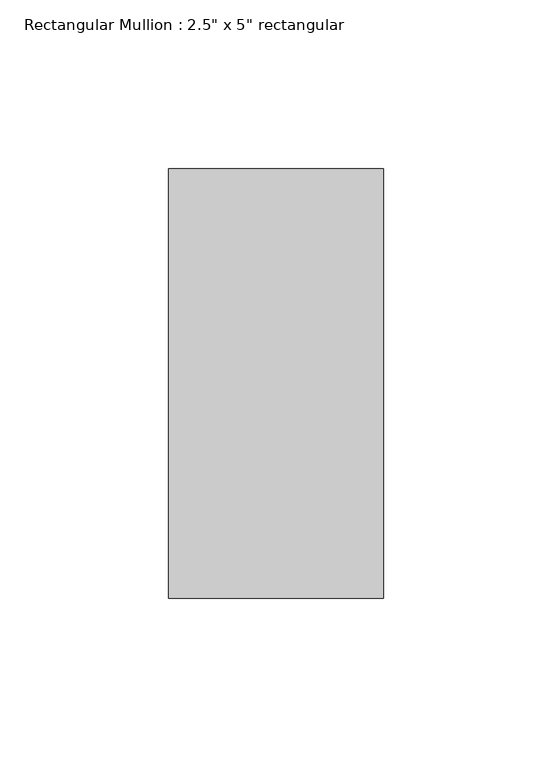
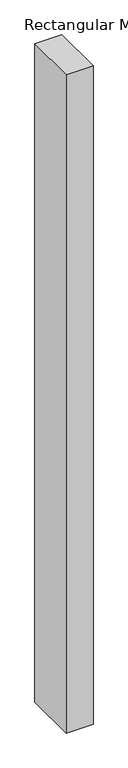
"""IFC4 building model written with IfcOpenShell, lengths in millimetres: member geometry."""

from ifc_helpers import new_model, si_unit, frame, origin, place, context, project, spatial, polyline, outline, extrude, source, transform, mapped, element, save


def member_f6b14484(model_context):
    return source(origin(), model_context, "Body", "SweptSolid", [
        extrude(outline(polyline([(0.0, 63.5), (0.0, -63.5), (-63.5, -63.5), (-63.5, 63.5), (0.0, 63.5)])), frame((0.0, 0.0, -1636.844519), z_axis=(0.0, 0.0, 1.0), x_axis=(1.0, 0.0, 0.0)), (0.0, 0.0, 1.0), 1636.844519),
    ])


if __name__ == "__main__":
    model = new_model("IFC4")
    model_context = context("Model", 3, world=origin())
    ifc_project = project(units=[si_unit("LENGTHUNIT", "METRE", prefix="MILLI")], contexts=[model_context])
    site = spatial("IfcSite", under=ifc_project)
    building = spatial("IfcBuilding", under=site)
    placement = place(None, origin())
    member_shape = member_f6b14484(model_context)
    element("IfcMember", 1, ObjectType="Rectangular Mullion : 2.5\" x 5\" rectangular", at=placement, inside=building, context=model_context, shape_type="MappedRepresentation", body=[
        mapped(member_shape, transform((0.0, 0.0, 0.0), x_axis=(1.0, 0.0, 0.0), y_axis=(0.0, 1.0, 0.0), z_axis=(0.0, 0.0, 1.0))),
    ])
    save(model, "model.ifc")

# Revit data of these elements
# Type "Rectangular Mullion : 2.5\" x 5\" rectangular"
#   built-in parameter 1007304 = 0.416667 (stored number, unit not read)
#   built-in parameter 1007301 = 0.104167 (stored number, unit not read)
#   built-in parameter 1007300 = 0.104167 (stored number, unit not read)
# Element 1 (IfcMember, "Rectangular Mullion : 2.5\" x 5\" rectangular")
#   Materials on its faces: "Aluminum"
# Materials
#   "Aluminum": class "Metal", colour RGB 247 247 247, transparency 0, Description = "Aluminum 6061", Cost = 0
